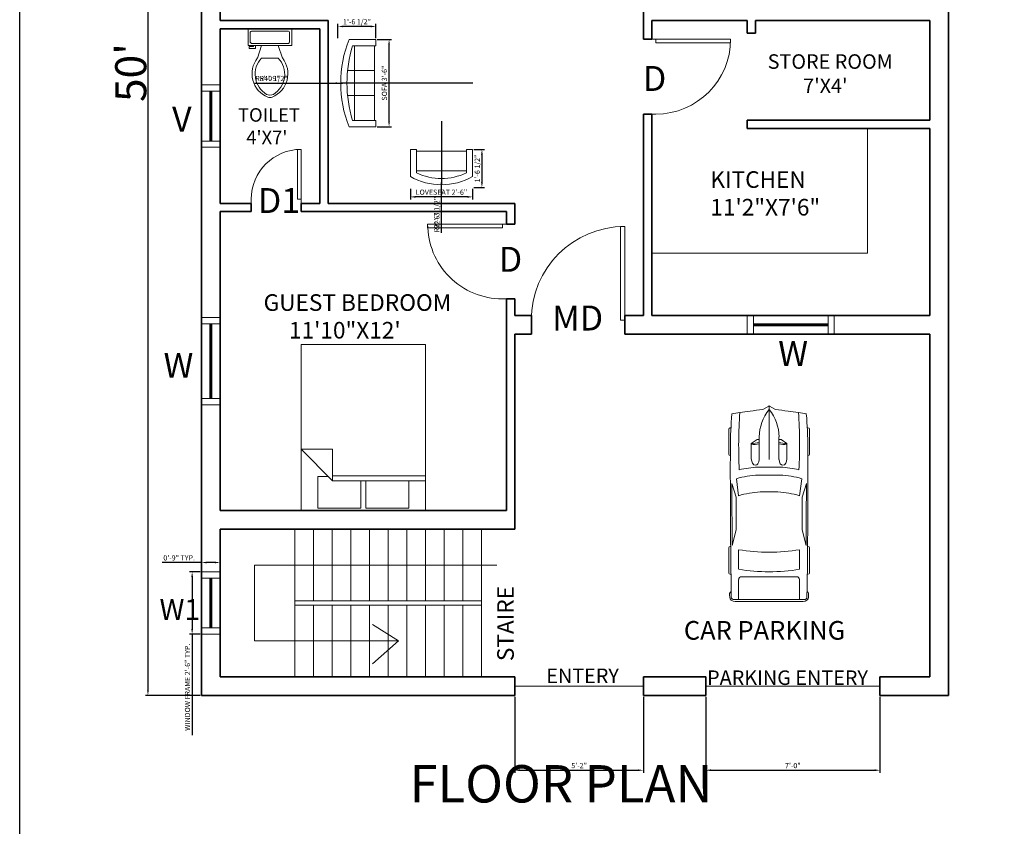
# Model space of a CAD drawing. Units: inches. Extents: x 2169 to 10664, y 1669 to 6352.
# Tile 3 of 17: x 2169 to 2644, y 2091 to 2480. Entities that reach past the tile are written whole.
import ezdxf

# ---------------------------------------------------------------- set-up
doc = ezdxf.new("R2010")
doc.units = ezdxf.units.IN
for name, color, linetype, lineweight in [('A-ANNO-DIMS', 3, 'Continuous', 18), ('A-ANNO-IDEN', 3, 'Continuous', 18), ('A-ANNO-SYMB', 6, 'Continuous', 13), ('A-ANNO-TITL', 3, 'Continuous', 25), ('A-ANNO-TTLB', 7, 'Continuous', 25), ('A-AREA-IDEN', 4, 'Continuous', 18), ('A-DOOR', 4, 'Continuous', 18), ('A-EQPM', 8, 'Continuous', 18), ('A-FLOR-CASE', 8, 'Continuous', 18), ('A-FLOR-FIXT', 9, 'Continuous', 18), ('A-FLOR-STRS', 4, 'Continuous', 18), ('A-FURN', 8, 'Continuous', 18), ('A-GLAZ', 30, 'Continuous', 18), ('A-WALL', 7, 'Continuous', 35)]:
    doc.layers.add(name, color=color, linetype=linetype, lineweight=lineweight)
doc.styles.get("Standard").update_dxf_attribs({"font": 'arial.ttf'})
doc.dimstyles.new('ISO-25', dxfattribs={"dimtxt": 2.5, "dimasz": 2.5, "dimexe": 1.25, "dimexo": 0.625, "dimtad": 1, "dimdec": 0, "dimlunit": 3, "dimtxsty": 'Standard', "dimcen": 2.5, "dimadec": 0, "dimazin": 0, "dimtfac": 1, "dimtdec": 0, "dimtmove": 0, "dimatfit": 3, "dimfxl": 1, "dimarcsym": 0})

# ---------------------------------------------------------------- blocks, each defined once
blk = doc.blocks.new('*U2')
for p, q in [((0, 0), (0, -6)), ((-40, 0), (-40, -6))]:
    blk.add_line(p, q)
blk.add_lwpolyline([(0, 0), (0, 40), (-1.75, 40), (-1.75, 0)], close=True)
blk.add_arc((0, 0), 40, 90, 180)
blk = doc.blocks.new('*U3')
for p, q in [((-24, 0), (-24, -6)), ((0, 0), (0, -6))]:
    blk.add_line(p, q)
blk.add_lwpolyline([(0, 0), (0, 24), (-1.75, 24), (-1.75, 0)], close=True)
blk.add_arc((0, 0), 24, 90, 180)
blk = doc.blocks.new('*U4')
for p, q in [((0, 0), (0, -6)), ((36, 0), (36, -6))]:
    blk.add_line(p, q)
blk.add_lwpolyline([(0, 0), (0, 36), (1.75, 36), (1.75, 0)], close=True)
blk.add_arc((0, 0), 36, 0, 90)
blk = doc.blocks.new('Toilet - top')
for p, q in [((9.5, -6), (9.5, -2)), ((-10, -8.5), (-8, -8.5)), ((-10, -9.5), (-10, -8.5)), ((-8, -8.5), (-8, -8)), ((-7, -8), (-7, -9.5)), ((-4, -8), (-6, -14)), ((4, -8), (6, -14)), ((-7, -9.5), (-10, -9.5)), ((4, -14), (-4, -14))]:
    blk.add_line(p, q)
blk.add_lwpolyline([(10.5, -8), (10.5, 0), (-10.5, 0), (-10.5, -8)], close=True)
for points in [[(-9.5, -2), (-9.5, -6)], [(8.5, -1), (-8.5, -1)], [(-8.5, -7), (8.5, -7)]]:
    blk.add_lwpolyline(points)
for centre, radius, start, end in [((-8.62, -1.88), 0.884, 81.8699, 188.1301), ((8.62, -1.88), 0.884, 351.8699, 98.1301), ((-8.62, -6.12), 0.884, 171.8699, 278.1301), ((8.62, -6.12), 0.884, 261.8699, 8.1301), ((3.52, -21.58), 12.17, 141.4691, 247.9714), ((4.2, -21.82), 11.33, 136.3677, 238.9468), ((-3.52, -21.58), 12.17, 292.0284, 38.5307), ((-4.2, -21.82), 11.33, 301.053, 43.6321), ((0, -27.88), 4, 245.7318, 294.2682), ((0, -29), 4, 254.8605, 285.1395)]:
    blk.add_arc(centre, radius, start, end)
blk = doc.blocks.new('Bed - Queen')
for p, q in [((0, -80.00003), (0, 0)), ((0, 0), (59.99999, 0)), ((59.99999, 0), (59.99999, -80.00003)), ((7.99999, -1.2), (28.79998, -1.2)), ((7.99999, -14.4), (7.99999, -1.2)), ((28.79998, -1.2), (28.79998, -14.4)), ((31.19999, -1.2), (51.99999, -1.2)), ((31.19999, -14.4), (31.19999, -1.2)), ((51.99999, -1.2), (51.99999, -16.4)), ((0, -14.4), (44.8, -14.4)), ((44.8, -16.8), (0, -16.8)), ((59.99999, -29.6), (44.8, -14.4)), ((44.8, -14.4), (44.8, -29.6)), ((51.99999, -16.4), (46.79936, -16.4)), ((44.8, -29.6), (59.99999, -29.6)), ((59.99999, -80.00003), (0, -80.00003))]:
    blk.add_line(p, q)
blk = doc.blocks.new('Sofa - Roundback 7 ft.')
for p, q in [((-12.00002, -32.4421), (-12.00003, -6.5971)), ((11.99997, -32.4421), (11.99998, -6.5971)), ((-36.000027, -34), (-36.000027, -11.4696)), ((-35.999844, -13.3819), (35.9998, -13.3819)), ((35.99998, -34), (35.99998, -11.4696)), ((-36.000027, -32.4421), (35.99998, -32.4421))]:
    blk.add_line(p, q)
for points in [[(-36.000027, -34), (-42.000027, -34), (-42.000027, -8)], [(41.99998, -8), (41.99998, -34), (35.99998, -34)]]:
    blk.add_lwpolyline(points)
for centre, radius, start, end in [((0, -114.25), 114.25, 68.43141, 111.5686), ((-0.00001, -127.1968), 121.1968, 72.72033, 107.2797)]:
    blk.add_arc(centre, radius, start, end)
blk = doc.blocks.new('Sofa - Roundback Loveseat 5 ft.')
for p, q in [((0, -32.44198), (0, -5.99998)), ((-24, -33.99998), (-24, -11.46958)), ((-23.9998, -13.38178), (23.99986, -13.38178)), ((24.00004, -33.99998), (24.00004, -11.46958)), ((-24, -32.44198), (24.00004, -32.44198))]:
    blk.add_line(p, q)
for points in [[(-24, -33.99998), (-30, -33.99998), (-30, -7.99998)], [(30.00004, -7.99998), (30.00004, -33.99998), (24.00004, -33.99998)]]:
    blk.add_lwpolyline(points)
for centre, radius, start, end in [((0, -60.24998), 60.24998, 60.13715, 119.8628), ((0, -61.38438), 55.38444, 64.32083, 115.6792)]:
    blk.add_arc(centre, radius, start, end)
blk = doc.blocks.new('*U16')
for p, q in [((0, 0), (0, 6)), ((36, 0), (36, 6))]:
    blk.add_line(p, q)
blk.add_lwpolyline([(0, 0), (0, -36), (1.75, -36), (1.75, 0)], close=True)
blk.add_arc((0, 0), 36, 270, 0)
blk = doc.blocks.new('*U18')
for p, q in [((1182, 988), (568, 988)), ((3472, 988), (4087, 988)), ((536, 950), (536, 936)), ((1214, 950), (1214, 950)), ((1779, 801), (2195, 746)), ((2235, 810), (1899, 912)), ((3412, 904), (3030, 807)), ((3440, 942), (3440, 950)), ((3516, 746), (3994, 746)), ((4119, 950), (4119, 934)), ((4736, 746), (4242, 746)), ((4736, -851), (4736, 851)), ((4785, -832), (4785, 832)), ((4179, 670), (4179, -670)), ((756, 241), (1313, 241)), ((816, 241), (816, 283)), ((820, 295), (918, 436)), ((918, 436), (1294, 436)), ((1496, -274), (1496, 274)), ((1690, -267), (1690, 267)), ((4736, -267), (4736, 267)), ((83, 156), (3, 10)), ((2102, 216), (2102, -216)), ((0, 0), (1313, 0)), ((3, -10), (83, -156)), ((756, -241), (1313, -241)), ((816, -241), (816, -283)), ((820, -295), (918, -436)), ((918, -436), (1294, -436)), ((536, -950), (536, -936)), ((1214, -950), (1214, -950)), ((2195, -746), (1779, -801)), ((2235, -810), (1899, -912)), ((3412, -904), (3030, -807)), ((3440, -942), (3440, -950)), ((3994, -746), (3516, -746)), ((4119, -950), (4119, -934)), ((4242, -746), (4736, -746)), ((1182, -988), (568, -988)), ((3472, -988), (4087, -988))]:
    blk.add_line(p, q)
for centre, major_axis, ratio, start_param, end_param in [((568, 950), (0, -37.6), 0.842304, 3.141593, 4.712389), ((1182, 950), (0, 37.6), 0.842304, -1.570796, 0), ((3472, 950), (0, -37.6), 0.842304, 3.141593, 4.712389), ((4087, 950), (0, 37.6), 0.842304, -1.570796, 0), ((4588, 910), (0, 56.4), 0.842304, -0.013017, 1.249894), ((1638, -268131), (0, 269121), 0.842304, -0.013397, -0.013017), ((4673, 832), (0, -133), 0.842304, 1.570796, 3.128196), ((6757, -699), (0, 7958), 0.842304, 1.367076, 1.39176), ((952, -15087), (0, -15833), 0.842304, 3.096046, 3.200911), ((1046, -12468), (0, 13417), 0.842304, 0.00281, 0.075598), ((1638, -268113), (0, 269063), 0.842304, -0.013397, 0.002797), ((3414, 137), (0, -2280), 0.842304, 4.449482, 4.652344), ((3436, 137), (0, 2077), 0.842304, 1.245306, 1.50788), ((1638, -268113), (0, -269025), 0.842304, 3.133765, 3.140441), ((3800, 71), (0, -2021), 0.842304, 4.372215, 4.640744), ((2433, -93125), (0, -93935), 0.842304, 3.134049, 3.144098), ((434, 0), (0, 3734), 0.842304, 4.511394, 4.913384), ((912, 0), (0, 3734), 0.842304, 4.511394, 4.913384), ((4242, 670), (0, 75.2), 0.842304, 0, 1.570796), ((4673, 851), (0, -75.2), 0.842304, 1.570796, 3.128196), ((6583, -699), (0, -7755), 0.842304, 4.528606, 4.561838), ((-5194, 1331), (0, -6374), 0.842304, 1.385369, 1.434372), ((756, -1185), (0, 1427), 0.842304, 0, 0.590319), ((832, 283), (0, 18.8), 0.842304, 0.879714, 1.570796), ((331, 432), (0, 696), 0.842304, 4.435146, 4.718221), ((361, 432), (0, 696), 0.842304, 4.435146, 4.718221), ((1290, 339), (161, -9), 0.603834, -1.395552, 1.581315), ((16, 0), (0, -18.8), 0.842304, 4.131459, 5.293319), ((-5194, -1331), (0, 6374), 0.842304, -1.434372, -1.385369), ((756, 1185), (0, 1427), 0.842304, 2.551274, 3.141593), ((3800, -71), (0, -2021), 0.842304, -1.499151, -1.230623), ((6583, 699), (0, 7755), 0.842304, 1.721348, 1.754579), ((832, -283), (0, -18.8), 0.842304, 4.712389, 5.403472), ((331, -432), (0, -696), 0.842304, 1.564964, 1.848039), ((361, -432), (0, -696), 0.842304, 1.564964, 1.848039), ((3414, -137), (0, -2280), 0.842304, -1.510751, -1.307889), ((3436, -137), (0, -2077), 0.842304, -1.50788, -1.245306), ((6757, 699), (0, 7958), 0.842304, 1.749832, 1.774517), ((952, 15087), (0, -15833), 0.842304, -0.059319, 0.045547), ((4242, -670), (0, -75.2), 0.842304, 4.712389, 6.283185), ((1046, 12468), (0, -13417), 0.842304, -0.075598, -0.00281), ((568, -950), (0, 37.6), 0.842304, 1.570796, 3.141593), ((1638, 268113), (0, 269063), 0.842304, 3.138796, 3.15499), ((1182, -950), (0, -37.6), 0.842304, 0, 1.570796), ((1638, 268113), (0, -269025), 0.842304, 0.001152, 0.007828), ((2433, 93125), (0, -93935), 0.842304, -0.002505, 0.007544), ((3472, -950), (0, -37.6), 0.842304, -1.570796, 0), ((4087, -950), (0, 37.6), 0.842304, 3.141593, 4.712389), ((4588, -910), (0, -56.4), 0.842304, -1.249894, 0.013017), ((4673, -851), (0, 75.2), 0.842304, 3.15499, 4.712389), ((4673, -832), (0, -133), 0.842304, 0.013397, 1.570796), ((1638, 268131), (0, 269121), 0.842304, 3.15461, 3.15499)]:
    blk.add_ellipse(centre, major_axis=major_axis, ratio=ratio, start_param=start_param, end_param=end_param)
at = {"extrusion": (0, 0, -1)}
blk.add_ellipse((1290, -339), major_axis=(161, 9), ratio=0.603834, start_param=-1.395552, end_param=1.581315, dxfattribs=at)
blk = doc.blocks.new('*D20')
at = {"layer": 'A-ANNO-DIMS', "color": 0, "lineweight": -2, "transparency": 16777216}
for p, q in [((2256.43, 2754.23), (2230.01, 2754.23)), ((2231.26, 2751.73), (2231.26, 2156.73)), ((2256.43, 2154.23), (2230.01, 2154.23))]:
    blk.add_line(p, q, dxfattribs=at)
at = {"layer": 'A-ANNO-DIMS', "color": 0, "transparency": 16777216}
for points in [[(2230.85, 2751.73), (2231.68, 2751.73), (2231.26, 2754.23)], [(2230.85, 2156.73), (2231.68, 2156.73), (2231.26, 2154.23)]]:
    blk.add_solid(points, dxfattribs=at)
at = {"layer": 'Defpoints', "color": 0, "transparency": 16777216}
for p in [(2257.06, 2754.23), (2231.26, 2154.23), (2257.06, 2154.23)]:
    blk.add_point(p, dxfattribs=at)
at = {"layer": 'A-ANNO-DIMS', "color": 0, "transparency": 16777216, "insert": (2222.98, 2454.23), "char_height": 2.5, "attachment_point": 5, "rotation": 90}
blk.add_mtext("{\\H6x;50'}", dxfattribs=at)
blk = doc.blocks.new('WIN-36-WALL-9')
for p, q in [((9, 42), (0, 42)), ((9, 39), (0, 39)), ((4, 39), (4, 3)), ((4.5, 39), (4.5, 3)), ((5, 39), (5, 3)), ((9, 3), (0, 3)), ((9, 0), (0, 0))]:
    blk.add_line(p, q)
blk = doc.blocks.new('WIN-24-WALL-9')
for p, q in [((9, 30), (0, 30)), ((9, 27), (0, 27)), ((4, 27), (4, 3)), ((4.5, 27), (4.5, 3)), ((5, 27), (5, 3)), ((9, 3), (0, 3)), ((9, 0), (0, 0))]:
    blk.add_line(p, q)
blk = doc.blocks.new('*D57')
at = {"layer": 'A-ANNO-DIMS', "color": 0, "lineweight": -2, "transparency": 16777216}
for p, q in [((2256.43, 2213.73), (2251.31, 2213.73)), ((2252.56, 2211.23), (2252.56, 2186.23)), ((2256.43, 2183.73), (2251.31, 2183.73)), ((2252.56, 2183.73), (2252.56, 2135.15))]:
    blk.add_line(p, q, dxfattribs=at)
at = {"layer": 'A-ANNO-DIMS', "color": 0, "transparency": 16777216}
for points in [[(2252.14, 2211.23), (2252.98, 2211.23), (2252.56, 2213.73)], [(2252.14, 2186.23), (2252.98, 2186.23), (2252.56, 2183.73)]]:
    blk.add_solid(points, dxfattribs=at)
at = {"layer": 'Defpoints', "color": 0, "transparency": 16777216}
for p in [(2257.06, 2213.73), (2252.56, 2183.73), (2257.06, 2183.73)]:
    blk.add_point(p, dxfattribs=at)
at = {"layer": 'A-ANNO-DIMS', "color": 0, "transparency": 16777216, "insert": (2250.64, 2158.19), "char_height": 2.5, "attachment_point": 5, "rotation": 90}
blk.add_mtext('WINDOW FRAME 2\'-6" TYP.', dxfattribs=at)
blk = doc.blocks.new('*D58')
at = {"layer": 'A-ANNO-DIMS', "color": 0, "lineweight": -2, "transparency": 16777216}
for p, q in [((2257.06, 2218.23), (2238.07, 2218.23)), ((2257.06, 2214.36), (2257.06, 2219.48)), ((2263.56, 2218.23), (2259.56, 2218.23)), ((2266.06, 2214.36), (2266.06, 2219.48))]:
    blk.add_line(p, q, dxfattribs=at)
at = {"layer": 'A-ANNO-DIMS', "color": 0, "transparency": 16777216}
for points in [[(2259.56, 2218.65), (2259.56, 2217.82), (2257.06, 2218.23)], [(2263.56, 2218.65), (2263.56, 2217.82), (2266.06, 2218.23)]]:
    blk.add_solid(points, dxfattribs=at)
at = {"layer": 'Defpoints', "color": 0, "transparency": 16777216}
for p in [(2257.06, 2218.23), (2257.06, 2213.73), (2266.06, 2213.73)]:
    blk.add_point(p, dxfattribs=at)
at = {"layer": 'A-ANNO-DIMS', "color": 0, "transparency": 16777216, "insert": (2246.31, 2220.14), "char_height": 2.5, "attachment_point": 5}
blk.add_mtext('0\'-9" TYP.', dxfattribs=at)
blk = doc.blocks.new('*D61')
at = {"layer": 'A-ANNO-DIMS', "color": 0, "lineweight": -2, "transparency": 16777216}
for p, q in [((2341.79, 2470.13), (2348.72, 2470.13)), ((2347.47, 2430.63), (2347.47, 2467.63)), ((2341.79, 2428.13), (2348.72, 2428.13))]:
    blk.add_line(p, q, dxfattribs=at)
at = {"layer": 'A-ANNO-DIMS', "color": 0, "transparency": 16777216}
for points in [[(2347.05, 2467.63), (2347.88, 2467.63), (2347.47, 2470.13)], [(2347.05, 2430.63), (2347.88, 2430.63), (2347.47, 2428.13)]]:
    blk.add_solid(points, dxfattribs=at)
at = {"layer": 'Defpoints', "color": 0, "transparency": 16777216}
for p in [(2341.17, 2470.13), (2347.47, 2470.13), (2341.17, 2428.13)]:
    blk.add_point(p, dxfattribs=at)
at = {"layer": 'A-ANNO-DIMS', "color": 0, "transparency": 16777216, "insert": (2345.55, 2449.13), "char_height": 2.5, "attachment_point": 5, "rotation": 90}
blk.add_mtext('SOFA 3\'-6"', dxfattribs=at)
blk = doc.blocks.new('*D62')
at = {"layer": 'A-ANNO-DIMS', "color": 0, "lineweight": -2, "transparency": 16777216}
for p, q in [((2322.83, 2470.75), (2322.83, 2477.68)), ((2341.17, 2470.75), (2341.17, 2477.68)), ((2338.67, 2476.43), (2325.33, 2476.43))]:
    blk.add_line(p, q, dxfattribs=at)
at = {"layer": 'A-ANNO-DIMS', "color": 0, "transparency": 16777216}
for points in [[(2325.33, 2476.85), (2325.33, 2476.01), (2322.83, 2476.43)], [(2338.67, 2476.85), (2338.67, 2476.01), (2341.17, 2476.43)]]:
    blk.add_solid(points, dxfattribs=at)
at = {"layer": 'Defpoints', "color": 0, "transparency": 16777216}
for p in [(2322.83, 2476.43), (2322.83, 2470.13), (2341.17, 2470.13)]:
    blk.add_point(p, dxfattribs=at)
at = {"layer": 'A-ANNO-DIMS', "color": 0, "transparency": 16777216, "insert": (2332, 2478.35), "char_height": 2.5, "attachment_point": 5}
blk.add_mtext('1\'-6 1/2"', dxfattribs=at)
blk = doc.blocks.new('*D65')
at = {"layer": 'A-ANNO-DIMS', "color": 0, "lineweight": -2, "transparency": 16777216}
for p, q in [((2357.72, 2398.21), (2357.72, 2393.09)), ((2387.72, 2398.21), (2387.72, 2393.09)), ((2385.22, 2394.34), (2360.22, 2394.34))]:
    blk.add_line(p, q, dxfattribs=at)
at = {"layer": 'A-ANNO-DIMS', "color": 0, "transparency": 16777216}
for points in [[(2360.22, 2394.76), (2360.22, 2393.92), (2357.72, 2394.34)], [(2385.22, 2394.76), (2385.22, 2393.92), (2387.72, 2394.34)]]:
    blk.add_solid(points, dxfattribs=at)
at = {"layer": 'Defpoints', "color": 0, "transparency": 16777216}
for p in [(2357.72, 2398.84), (2387.72, 2398.84), (2357.72, 2394.34)]:
    blk.add_point(p, dxfattribs=at)
at = {"layer": 'A-ANNO-DIMS', "color": 0, "transparency": 16777216, "insert": (2372.72, 2396.26), "char_height": 2.5, "attachment_point": 5}
blk.add_mtext('LOVESEAT 2\'-6"', dxfattribs=at)
blk = doc.blocks.new('*D66')
at = {"layer": 'A-ANNO-DIMS', "color": 0, "lineweight": -2, "transparency": 16777216}
for p, q in [((2388.35, 2417.17), (2393.47, 2417.17)), ((2392.22, 2414.67), (2392.22, 2401.34)), ((2388.35, 2398.84), (2393.47, 2398.84))]:
    blk.add_line(p, q, dxfattribs=at)
at = {"layer": 'A-ANNO-DIMS', "color": 0, "transparency": 16777216}
for points in [[(2391.81, 2414.67), (2392.64, 2414.67), (2392.22, 2417.17)], [(2391.81, 2401.34), (2392.64, 2401.34), (2392.22, 2398.84)]]:
    blk.add_solid(points, dxfattribs=at)
at = {"layer": 'Defpoints', "color": 0, "transparency": 16777216}
for p in [(2387.72, 2417.17), (2387.72, 2398.84), (2392.22, 2398.84)]:
    blk.add_point(p, dxfattribs=at)
at = {"layer": 'A-ANNO-DIMS', "color": 0, "transparency": 16777216, "insert": (2390.31, 2408.01), "char_height": 2.5, "attachment_point": 5, "rotation": 90}
blk.add_mtext('1\'-6 1/2"', dxfattribs=at)
blk = doc.blocks.new('*D128')
at = {"layer": 'A-ANNO-DIMS', "color": 0, "lineweight": -2, "transparency": 16777216}
for p, q in [((2408.06, 2153.61), (2408.06, 2116.93)), ((2470.06, 2153.61), (2470.06, 2116.93)), ((2410.56, 2118.18), (2467.56, 2118.18))]:
    blk.add_line(p, q, dxfattribs=at)
at = {"layer": 'A-ANNO-DIMS', "color": 0, "transparency": 16777216}
for points in [[(2410.56, 2118.6), (2410.56, 2117.77), (2408.06, 2118.18)], [(2467.56, 2118.6), (2467.56, 2117.77), (2470.06, 2118.18)]]:
    blk.add_solid(points, dxfattribs=at)
at = {"layer": 'Defpoints', "color": 0, "transparency": 16777216}
for p in [(2408.06, 2154.23), (2470.06, 2154.23), (2470.06, 2118.18)]:
    blk.add_point(p, dxfattribs=at)
at = {"layer": 'A-ANNO-DIMS', "color": 0, "transparency": 16777216, "insert": (2439.06, 2120.09), "char_height": 2.5, "attachment_point": 5}
blk.add_mtext('5\'-2"', dxfattribs=at)
blk = doc.blocks.new('*D129')
at = {"layer": 'A-ANNO-DIMS', "color": 0, "lineweight": -2, "transparency": 16777216}
for p, q in [((2500.06, 2153.61), (2500.06, 2116.93)), ((2584.06, 2153.61), (2584.06, 2116.93)), ((2502.56, 2118.18), (2581.56, 2118.18))]:
    blk.add_line(p, q, dxfattribs=at)
at = {"layer": 'A-ANNO-DIMS', "color": 0, "transparency": 16777216}
for points in [[(2502.56, 2118.6), (2502.56, 2117.77), (2500.06, 2118.18)], [(2581.56, 2118.6), (2581.56, 2117.77), (2584.06, 2118.18)]]:
    blk.add_solid(points, dxfattribs=at)
at = {"layer": 'Defpoints', "color": 0, "transparency": 16777216}
for p in [(2500.06, 2154.23), (2584.06, 2154.23), (2584.06, 2118.18)]:
    blk.add_point(p, dxfattribs=at)
at = {"layer": 'A-ANNO-DIMS', "color": 0, "transparency": 16777216, "insert": (2542.06, 2120.09), "char_height": 2.5, "attachment_point": 5}
blk.add_mtext('7\'-0"', dxfattribs=at)
blk = doc.blocks.new('*D130')
at = {"layer": 'A-ANNO-DIMS', "color": 0, "lineweight": -2, "transparency": 16777216}
for p, q in [((2282.75, 2449.13), (2324.67, 2449.13)), ((2387.77, 2449.13), (2327.17, 2449.13))]:
    blk.add_line(p, q, dxfattribs=at)
at = {"layer": 'A-ANNO-DIMS', "color": 0, "transparency": 16777216}
blk.add_solid([(2324.67, 2449.55), (2324.67, 2448.71), (2327.17, 2449.13)], dxfattribs=at)
at = {"layer": 'Defpoints', "color": 0, "transparency": 16777216}
for p in [(2327.17, 2449.13), (2387.77, 2449.13)]:
    blk.add_point(p, dxfattribs=at)
at = {"layer": 'A-ANNO-DIMS', "color": 0, "transparency": 16777216, "insert": (2290.81, 2451.05), "char_height": 2.5, "attachment_point": 5, "rotation": 359.9996}
blk.add_mtext('R5\'-0 1/2"', dxfattribs=at)
blk = doc.blocks.new('*D131')
at = {"layer": 'A-ANNO-DIMS', "color": 0, "lineweight": -2, "transparency": 16777216}
for p, q in [((2284.75, 2449.13), (2321.67, 2449.13)), ((2381.29, 2449.13), (2324.17, 2449.13))]:
    blk.add_line(p, q, dxfattribs=at)
at = {"layer": 'A-ANNO-DIMS', "color": 0, "transparency": 16777216}
blk.add_solid([(2321.67, 2449.55), (2321.67, 2448.71), (2324.17, 2449.13)], dxfattribs=at)
at = {"layer": 'Defpoints', "color": 0, "transparency": 16777216}
for p in [(2324.17, 2449.13), (2381.29, 2449.13)]:
    blk.add_point(p, dxfattribs=at)
at = {"layer": 'A-ANNO-DIMS', "color": 0, "transparency": 16777216, "insert": (2289.89, 2451.03), "char_height": 2.5, "attachment_point": 5, "rotation": 359.9996}
blk.add_mtext('R4\'-9"', dxfattribs=at)
blk = doc.blocks.new('*D132')
at = {"layer": 'A-ANNO-DIMS', "color": 0, "lineweight": -2, "transparency": 16777216}
for p, q in [((2372.72, 2430.3), (2372.72, 2400.17)), ((2372.72, 2376.95), (2372.72, 2397.67))]:
    blk.add_line(p, q, dxfattribs=at)
at = {"layer": 'A-ANNO-DIMS', "color": 0, "transparency": 16777216}
blk.add_solid([(2372.31, 2397.67), (2373.14, 2397.67), (2372.72, 2400.17)], dxfattribs=at)
at = {"layer": 'Defpoints', "color": 0, "transparency": 16777216}
for p in [(2372.72, 2430.3), (2372.72, 2400.17)]:
    blk.add_point(p, dxfattribs=at)
at = {"layer": 'A-ANNO-DIMS', "color": 0, "transparency": 16777216, "insert": (2370.82, 2382.1), "char_height": 2.5, "attachment_point": 5, "rotation": 89.9997}
blk.add_mtext('R2\'-6"', dxfattribs=at)
blk = doc.blocks.new('*D133')
at = {"layer": 'A-ANNO-DIMS', "color": 0, "lineweight": -2, "transparency": 16777216}
for p, q in [((2372.72, 2430.86), (2372.72, 2403.17)), ((2372.72, 2378.5), (2372.72, 2400.67))]:
    blk.add_line(p, q, dxfattribs=at)
at = {"layer": 'A-ANNO-DIMS', "color": 0, "transparency": 16777216}
blk.add_solid([(2372.31, 2400.67), (2373.14, 2400.67), (2372.72, 2403.17)], dxfattribs=at)
at = {"layer": 'Defpoints', "color": 0, "transparency": 16777216}
for p in [(2372.72, 2430.86), (2372.72, 2403.17)]:
    blk.add_point(p, dxfattribs=at)
at = {"layer": 'A-ANNO-DIMS', "color": 0, "transparency": 16777216, "insert": (2370.81, 2386.56), "char_height": 2.5, "attachment_point": 5, "rotation": 89.9997}
blk.add_mtext('R2\'-3 1/2"', dxfattribs=at)

msp = doc.modelspace()

# ---------------------------------------------------------------- linework, layer by layer
at = {"layer": 'A-ANNO-SYMB'}
for p, q in [((2399.46, 2216.98), (2282.59, 2216.98)), ((2282.59, 2216.98), (2282.59, 2180.48)), ((2352.06, 2180.48), (2339.44, 2188.44)), ((2282.59, 2180.48), (2352.06, 2180.48)), ((2352.06, 2180.48), (2339.44, 2169.43))]:
    msp.add_line(p, q, dxfattribs=at)
at = {"layer": 'A-ANNO-TTLB'}
msp.add_lwpolyline([(2169.45, 2838.28), (3251.13, 2838.28), (3251.13, 1669.34), (2169.45, 1669.34)], close=True, dxfattribs=at)
at = {"layer": 'A-DOOR'}
for p, q in [((2408.06, 2158.73), (2470.06, 2158.73)), ((2500.06, 2158.73), (2584.06, 2158.73))]:
    msp.add_line(p, q, dxfattribs=at)
at = {"layer": 'A-FLOR-CASE'}
for p in [(2578.06, 2427.23), (2474.06, 2367.23)]:
    msp.add_line(p, (2578.06, 2367.23), dxfattribs=at)
at = {"layer": 'A-FLOR-STRS'}
for p, q in [((2302.06, 2163.23), (2302.06, 2234.23)), ((2311.06, 2199.73), (2311.06, 2234.23)), ((2320.06, 2199.73), (2320.06, 2234.23)), ((2329.06, 2199.73), (2329.06, 2234.23)), ((2338.06, 2199.73), (2338.06, 2234.23)), ((2347.06, 2199.73), (2347.06, 2234.23)), ((2356.06, 2199.73), (2356.06, 2234.23)), ((2365.06, 2199.73), (2365.06, 2234.23)), ((2374.06, 2199.73), (2374.06, 2234.23)), ((2383.06, 2199.73), (2383.06, 2234.23)), ((2392.06, 2163.23), (2392.06, 2234.23)), ((2302.06, 2199.73), (2392.06, 2199.73)), ((2302.06, 2197.73), (2392.06, 2197.73)), ((2311.06, 2163.23), (2311.06, 2197.73)), ((2320.06, 2163.23), (2320.06, 2197.73)), ((2329.06, 2163.23), (2329.06, 2197.73)), ((2338.06, 2163.23), (2338.06, 2197.73)), ((2347.06, 2163.23), (2347.06, 2197.73)), ((2356.06, 2163.23), (2356.06, 2197.73)), ((2365.06, 2163.23), (2365.06, 2197.73)), ((2374.06, 2163.23), (2374.06, 2197.73)), ((2383.06, 2163.23), (2383.06, 2197.73))]:
    msp.add_line(p, q, dxfattribs=at)
at = {"layer": 'A-WALL'}
for p, q in [((2257.06, 2154.23), (2257.06, 2754.23)), ((2617.06, 2754.23), (2617.06, 2154.23)), ((2266.06, 2479.23), (2266.06, 2515.23)), ((2470.06, 2470.23), (2470.06, 2492.23)), ((2266.06, 2479.23), (2318.06, 2479.23)), ((2318.06, 2391.23), (2318.06, 2479.23)), ((2474.06, 2479.23), (2520.06, 2479.23)), ((2474.06, 2470.23), (2474.06, 2479.23)), ((2520.06, 2479.23), (2520.06, 2473.23)), ((2524.06, 2479.23), (2524.06, 2473.23)), ((2524.06, 2479.23), (2608.06, 2479.23)), ((2608.06, 2479.23), (2608.06, 2431.23)), ((2266.06, 2475.23), (2314.06, 2475.23)), ((2266.06, 2391.23), (2266.06, 2475.23)), ((2314.06, 2391.23), (2314.06, 2475.23)), ((2520.06, 2473.23), (2524.06, 2473.23)), ((2470.06, 2470.23), (2474.06, 2470.23)), ((2470.06, 2337.23), (2470.06, 2434.23)), ((2470.06, 2434.23), (2474.06, 2434.23)), ((2474.06, 2337.23), (2474.06, 2434.23)), ((2520.06, 2431.23), (2608.06, 2431.23)), ((2520.06, 2431.23), (2520.06, 2427.23)), ((2520.06, 2427.23), (2608.06, 2427.23)), ((2608.06, 2427.23), (2608.06, 2337.23)), ((2266.06, 2391.23), (2281.06, 2391.23)), ((2266.06, 2387.23), (2281.06, 2387.23)), ((2266.06, 2243.23), (2266.06, 2387.23)), ((2281.06, 2387.23), (2281.06, 2391.23)), ((2305.06, 2387.23), (2305.06, 2391.23)), ((2305.06, 2391.23), (2314.06, 2391.23)), ((2305.06, 2387.23), (2404.06, 2387.23)), ((2318.06, 2391.23), (2408.06, 2391.23)), ((2404.06, 2381.23), (2404.06, 2387.23)), ((2408.06, 2381.23), (2408.06, 2391.23)), ((2404.06, 2381.23), (2408.06, 2381.23)), ((2404.06, 2243.23), (2404.06, 2345.23)), ((2404.06, 2345.23), (2408.06, 2345.23)), ((2408.06, 2337.23), (2408.06, 2345.23)), ((2408.06, 2337.23), (2416.06, 2337.23)), ((2416.06, 2328.23), (2416.06, 2337.23)), ((2461.06, 2337.23), (2470.06, 2337.23)), ((2461.06, 2328.23), (2461.06, 2337.23)), ((2474.06, 2337.23), (2608.06, 2337.23)), ((2408.06, 2234.23), (2408.06, 2328.23)), ((2408.06, 2328.23), (2416.06, 2328.23)), ((2461.06, 2328.23), (2608.06, 2328.23)), ((2608.06, 2328.23), (2608.06, 2163.23)), ((2266.06, 2243.23), (2404.06, 2243.23)), ((2266.06, 2163.23), (2266.06, 2234.23)), ((2266.06, 2234.23), (2408.06, 2234.23)), ((2408.06, 2163.23), (2266.06, 2163.23)), ((2408.06, 2163.23), (2408.06, 2154.23)), ((2470.06, 2163.23), (2470.06, 2154.23)), ((2500.06, 2163.23), (2470.06, 2163.23)), ((2500.06, 2163.23), (2500.06, 2154.23)), ((2608.06, 2163.23), (2584.06, 2163.23)), ((2584.06, 2163.23), (2584.06, 2154.23)), ((2408.06, 2154.23), (2257.06, 2154.23)), ((2500.06, 2154.23), (2470.06, 2154.23)), ((2617.06, 2154.23), (2584.06, 2154.23))]:
    msp.add_line(p, q, dxfattribs=at)

# ---------------------------------------------------------------- block references
at = {"layer": 'A-DOOR', "rotation": 270}
for name, p in [('*U4', (2476.06, 2470.23)), ('*U16', (2402.06, 2381.23))]:
    msp.add_blockref(name, p, dxfattribs=at)
at = {"layer": 'A-DOOR'}
msp.add_blockref('*U3', (2305.06, 2393.23), dxfattribs=at)
at = {"layer": 'A-DOOR', "xscale": 1.127021996072997, "yscale": 1.127021996072997, "zscale": 1.127021996072997}
msp.add_blockref('*U2', (2461.06, 2335), dxfattribs=at)
at = {"layer": 'A-EQPM', "xscale": 0.0196850393700788, "yscale": 0.0196850393700788, "zscale": 0.0196850393700788, "rotation": 270}
msp.add_blockref('*U18', (2530.64, 2293.62), dxfattribs=at)
at = {"layer": 'A-FLOR-FIXT'}
msp.add_blockref('Toilet - top', (2290.06, 2475.23), dxfattribs=at)
at = {"layer": 'A-FURN', "xscale": 0.5, "yscale": 0.5, "zscale": 0.5}
for name, p, rotation in [('Sofa - Roundback 7 ft.', (2324.17, 2449.13), 90), ('Sofa - Roundback Loveseat 5 ft.', (2372.72, 2400.17), 180)]:
    msp.add_blockref(name, p, dxfattribs=dict(at, rotation=rotation))
at = {"layer": 'A-FURN', "rotation": 180}
msp.add_blockref('Bed - Queen', (2365.06, 2243.23), dxfattribs=at)
at = {"layer": 'A-GLAZ'}
for name, p, rotation in [('WIN-24-WALL-9', (2266.06, 2448.23), 180), ('WIN-36-WALL-9', (2266.06, 2336.23), 180), ('WIN-36-WALL-9', (2562.06, 2328.23), 90.0000000000021), ('WIN-24-WALL-9', (2266.06, 2213.73), 180)]:
    msp.add_blockref(name, p, dxfattribs=dict(at, rotation=rotation))

# ---------------------------------------------------------------- texts
at = {"layer": 'A-ANNO-IDEN', "attachment_point": 1}
for s, insert, char_height in [('D', (2469.81, 2457.37), 12), ('V', (2242.89, 2437.81), 12), ('D1', (2284.26, 2398.58), 12), ('D', (2400.37, 2370.26), 12), ('MD', (2426.08, 2341.97), 12), ('W', (2535.01, 2324.9), 12), ('W', (2238.78, 2319.22), 12), ('W1', (2236.85, 2200.61), 10)]:
    msp.add_mtext_dynamic_manual_height_columns(s, width=497.3673, gutter_width=12.5, heights=[0], dxfattribs=dict(at, insert=insert, char_height=char_height))
at = {"layer": 'A-ANNO-TITL', "insert": (2357.28, 2120.64), "char_height": 18, "attachment_point": 1}
msp.add_mtext_dynamic_manual_height_columns('FLOOR PLAN', width=979.1036, gutter_width=12.5, heights=[0], dxfattribs=at)
at = {"layer": 'A-AREA-IDEN', "attachment_point": 1}
for s, width, insert, char_height in [("STORE ROOM\\P        7'X4'", 172.6537, (2529.94, 2463.02), 7), ("TOILET\\P  4'X7'", 196.7478, (2274.67, 2437.06), 6.5), ('KITCHEN\\P11\'2"X7\'6"', 286.7524, (2502.29, 2406.69), 8), ('GUEST BEDROOM\\P     11\'10"X12\'', 906.8511, (2287, 2347.44), 8), ('CAR PARKING', 121.9344, (2489.55, 2190.06), 9), ('ENTERY', 101.3725, (2423.23, 2167.15), 7), ('PARKING ENTERY', 108.0021, (2500.75, 2166.26), 7)]:
    msp.add_mtext_dynamic_manual_height_columns(s, width=width, gutter_width=12.5, heights=[0], dxfattribs=dict(at, insert=insert, char_height=char_height))
at = {"layer": 'A-AREA-IDEN', "insert": (2399.59, 2170.72), "char_height": 8, "attachment_point": 1, "rotation": 90}
msp.add_mtext_dynamic_manual_height_columns('STAIRE', width=662.6127, gutter_width=12.5, heights=[0], dxfattribs=at)

# ---------------------------------------------------------------- dimensions: what is measured, and where the dimension line sits
at = {"layer": 'A-ANNO-DIMS'}
for base, p1, p2, angle, text, override, picture, middle in [((2231.26, 2154.23), (2257.06, 2754.23), (2257.06, 2154.23), 90, '{\\H6x;<>}', {"dimclrd": 0, "dimclre": 0, "dimclrt": 0}, '*D20', (2222.98, 2454.23)), ((2347.47, 2470.13), (2341.17, 2428.13), (2341.17, 2470.13), 90, 'SOFA <>', {"dimdec": 1, "dimlfac": 1, "dimrnd": 0, "dimzin": 1, "dimdsep": 46, "dimlunit": 4, "dimfrac": 2}, '*D61', (2345.55, 2449.13)), ((2357.72, 2394.34), (2387.72, 2398.84), (2357.72, 2398.84), 180, 'LOVESEAT <>', {"dimdec": 1, "dimlfac": 1, "dimrnd": 0, "dimzin": 1, "dimdsep": 46, "dimlunit": 4, "dimfrac": 2}, '*D65', (2372.72, 2396.26)), ((2257.06, 2218.23), (2266.06, 2213.73), (2257.06, 2213.73), 180, '<> TYP.', {"dimdec": 1, "dimlfac": 1, "dimrnd": 0, "dimzin": 1, "dimdsep": 46, "dimlunit": 4, "dimfrac": 2}, '*D58', (2246.31, 2220.14)), ((2252.56, 2183.73), (2257.06, 2213.73), (2257.06, 2183.73), 270, 'WINDOW FRAME <> TYP.', {"dimdec": 1, "dimlfac": 1, "dimrnd": 0, "dimzin": 1, "dimdsep": 46, "dimlunit": 4, "dimfrac": 2}, '*D57', (2250.64, 2158.19))]:
    dim = msp.add_linear_dim(base=base, p1=p1, p2=p2, angle=angle, text=text, dimstyle='ISO-25', override=override, dxfattribs=at)
    dim.commit()
    dim.dimension.update_dxf_attribs({"geometry": picture, "text_midpoint": middle})
for base, p1, p2, angle, picture, middle in [((2322.83, 2476.43), (2341.17, 2470.13), (2322.83, 2470.13), 180, '*D62', (2332, 2478.35)), ((2392.22, 2398.84), (2387.72, 2417.17), (2387.72, 2398.84), 270, '*D66', (2390.31, 2408.01))]:
    dim = msp.add_linear_dim(base=base, p1=p1, p2=p2, angle=angle, dimstyle='ISO-25', override={"dimdec": 1, "dimlfac": 1, "dimrnd": 0, "dimzin": 1, "dimdsep": 46, "dimlunit": 4, "dimfrac": 2}, dxfattribs=at)
    dim.commit()
    dim.dimension.update_dxf_attribs({"geometry": picture, "text_midpoint": middle})
for center, mpoint, picture, middle in [((2387.77, 2449.13), (2327.17, 2449.13), '*D130', (2290.81, 2449.13)), ((2381.29, 2449.13), (2324.17, 2449.13), '*D131', (2289.89, 2449.13)), ((2372.72, 2430.86), (2372.72, 2403.17), '*D133', (2372.72, 2386.56)), ((2372.72, 2430.3), (2372.72, 2400.17), '*D132', (2372.72, 2382.1))]:
    dim = msp.add_radius_dim(center=center, mpoint=mpoint, dimstyle='ISO-25', override={"dimdec": 1, "dimlfac": 1, "dimrnd": 0, "dimzin": 1, "dimdsep": 46, "dimlunit": 4, "dimfrac": 2}, dxfattribs=at)
    dim.commit()
    dim.dimension.update_dxf_attribs({"geometry": picture, "text_midpoint": middle, "dimtype": 164})
for base, p1, p2, picture, middle in [((2470.06, 2118.18), (2408.06, 2154.23), (2470.06, 2154.23), '*D128', (2439.06, 2120.09)), ((2584.06, 2118.18), (2500.06, 2154.23), (2584.06, 2154.23), '*D129', (2542.06, 2120.09))]:
    dim = msp.add_linear_dim(base=base, p1=p1, p2=p2, dimstyle='ISO-25', override={"dimdec": 1, "dimlfac": 1, "dimrnd": 0, "dimzin": 1, "dimdsep": 46, "dimlunit": 4, "dimfrac": 2}, dxfattribs=at)
    dim.commit()
    dim.dimension.update_dxf_attribs({"geometry": picture, "text_midpoint": middle})

doc.saveas('drawing.dxf')
